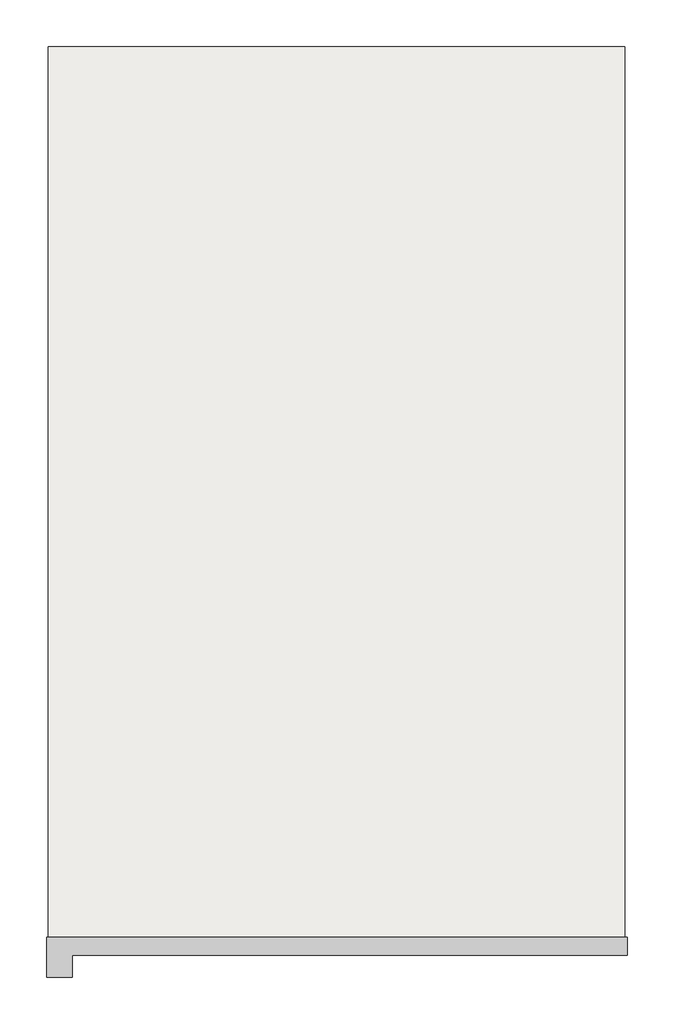
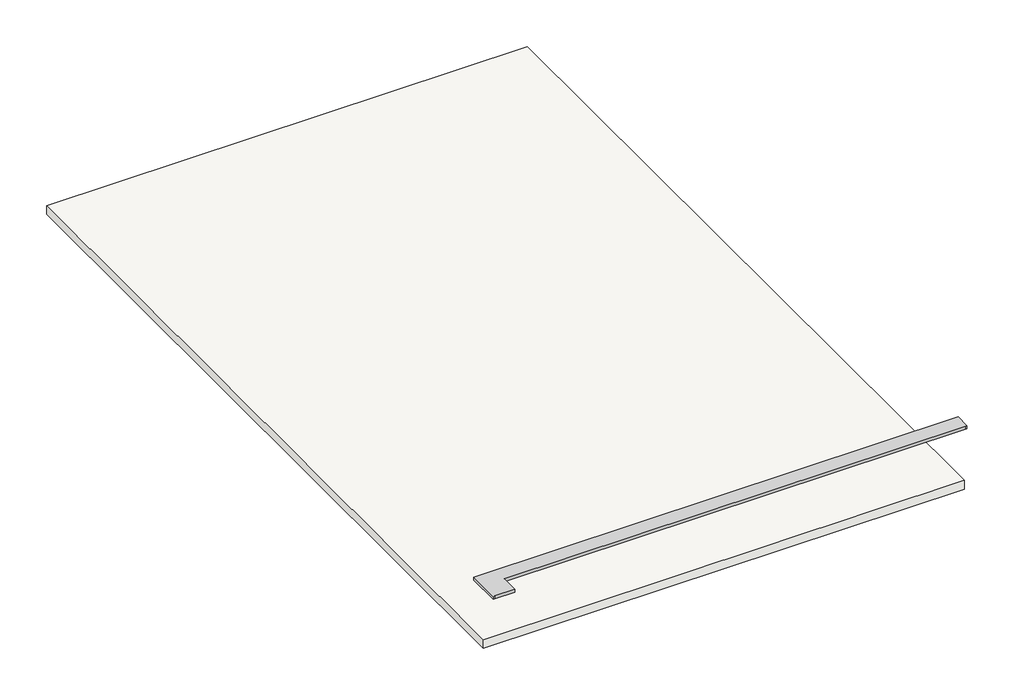
# One storey: 1 proxy, 1 slab.
"""IFC4 building model written with IfcOpenShell, lengths in millimetres."""

from ifc_helpers import new_model, si_unit, frame, origin, place, context, project, spatial, polyline, outline, extrude, transform, mapped, element, save
from components import generic_models_4_generic_models_4_4063ad9d

model = new_model("IFC4")

# Units and contexts
model_context = context("Model", 3, world=origin())
ifc_project = project(units=[si_unit("LENGTHUNIT", "METRE", prefix="MILLI")], contexts=[model_context])

# Site, building, storey
site = spatial("IfcSite", under=ifc_project)
building = spatial("IfcBuilding", under=site)
storey = spatial("IfcBuildingStorey", under=building, Elevation=7010.4)

# Proxy
placement = place(None, origin())
generic_models_4_generic_models_4_shape = generic_models_4_generic_models_4_4063ad9d(model_context)
element("IfcBuildingElementProxy", 1, Name="Generic Models 4 : Generic Models 4", ObjectType="Generic Models 4 : Generic Models 4", at=placement, inside=storey, context=model_context, shape_type="MappedRepresentation", body=[
    mapped(generic_models_4_generic_models_4_shape, transform((0.0, 0.0, 0.0), x_axis=(1.0, 0.0, 0.0), y_axis=(0.0, 1.0, 0.0), z_axis=(0.0, 0.0, 1.0))),
])

# Slab
element("IfcSlab", 2, ObjectType="SLAB 6\"", at=placement, inside=storey, context=model_context, shape_type="SweptSolid", body=[
    extrude(outline(polyline([(-506.5519453, 16519.6444012), (-506.5519453, 3972.0444012), (-8482.1519453, 3972.0444012), (-8482.1519453, 16519.6444012), (-506.5519453, 16519.6444012)])), frame((0.0, 0.0, 5943.6), z_axis=(0.0, 0.0, 1.0), x_axis=(1.0, 0.0, 0.0)), (0.0, 0.0, 1.0), 152.4),
])

save(model, "model.ifc")

# Revit data of these elements
# Type "SLAB 6\""
#   Assembly Code = "B1010"
#   Function = 0
#   Layers, outside or top first: 0' - 6" no material (function 1)
# Element 1 (IfcBuildingElementProxy, "Generic Models 4 : Generic Models 4")
#   Phase Created = New Construction
# Element 2 (IfcSlab, "SLAB 6\"")
#   Height Offset From Level = -3' - 0"
#   Phase Created = New Construction
#   Materials on its faces: "Default Floor"
# Materials
#   "Default Floor": colour RGB 128 128 128, transparency 0, Cost = 0
